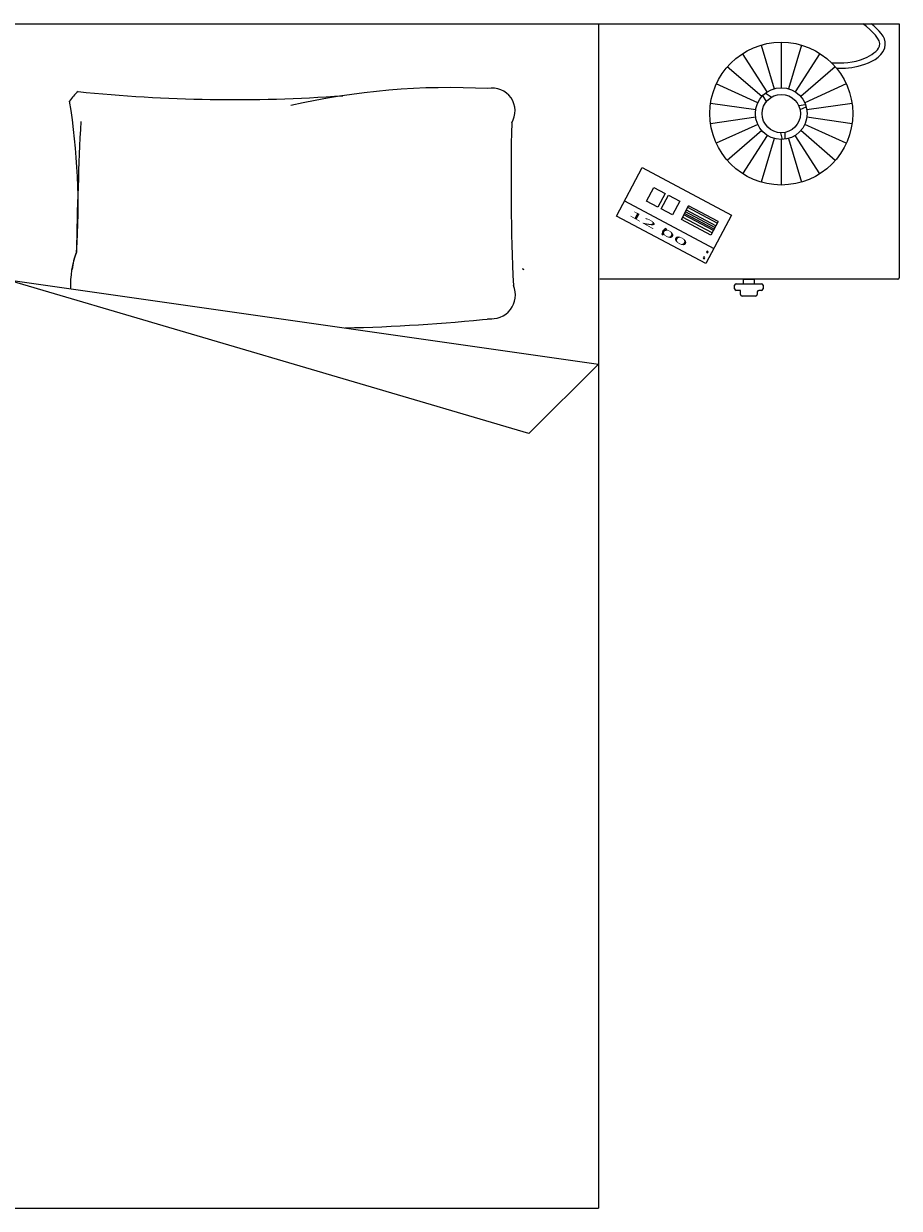
# Model space of a CAD drawing. Units: inches. Extents: x 1994 to 3075, y 3517 to 3950.
# Tile 8 of 58: x 1994.05149 to 1994.10437, y 3553.70967 to 3553.78125. Entities that reach past the tile are written whole.
import ezdxf

# ---------------------------------------------------------------- set-up
doc = ezdxf.new("R2010")
doc.units = ezdxf.units.IN
doc.layers.add('A-FURN-REFR', color=8, linetype='Continuous', lineweight=13)
doc.layers.add('A-FURN-REFR-TEXT', color=7, linetype='Continuous', lineweight=13)
doc.styles.get("Standard").update_dxf_attribs({"font": 'arial.ttf'})

msp = doc.modelspace()

# ---------------------------------------------------------------- linework, layer by layer
at = {"layer": 'A-FURN-REFR'}
for p, q in [((1994.014615338393, 3553.781253037129), (1994.086197299739, 3553.781253037129)), ((1994.086197299739, 3553.781253037129), (1994.10437051092, 3553.781253037129)), ((1994.086197299739, 3553.781253037129), (1994.10437051092, 3553.781253037129)), ((1994.086197299739, 3553.781253037129), (1994.086197299739, 3553.709671075784)), ((1994.10437051092, 3553.781253037129), (1994.10437051092, 3553.76590291077)), ((1994.096027345216, 3553.77996234353), (1994.096802931697, 3553.77732093855)), ((1994.097243416193, 3553.78013718814), (1994.097243416193, 3553.777384270659)), ((1994.097243416193, 3553.78013718814), (1994.097243416193, 3553.777384270659)), ((1994.098459487171, 3553.77996234353), (1994.09768390069, 3553.77732093855)), ((1994.096398132634, 3553.777136073012), (1994.094909793077, 3553.779451974569)), ((1994.09957703931, 3553.779451974569), (1994.098088699753, 3553.777136073012)), ((1994.096061813419, 3553.776844650753), (1994.093981297204, 3553.778647428315)), ((1994.100505535183, 3553.778647428315), (1994.098425018968, 3553.776844650753)), ((1994.095821220632, 3553.776470281071), (1994.093317078811, 3553.777613884321)), ((1994.101169753576, 3553.777613884321), (1994.098665611754, 3553.776470281071)), ((1994.096348791161, 3553.776556785599), (1994.096124540409, 3553.776912848794)), ((1994.096631392656, 3553.776804389888), (1994.096273766541, 3553.777047270305)), ((1994.095695845673, 3553.77604329317), (1994.092970948922, 3553.776435074175)), ((1994.098295634803, 3553.776305435665), (1994.09870586394, 3553.776373715132)), ((1994.098374763921, 3553.776069987851), (1994.098750731625, 3553.776236098163)), ((1994.101515883465, 3553.776435074175), (1994.098790986714, 3553.77604329317)), ((1994.095695845673, 3553.775598279071), (1994.092970948922, 3553.775206498065)), ((1994.101515883465, 3553.775206498065), (1994.098790986714, 3553.775598279071)), ((1994.095821220632, 3553.77517129117), (1994.093317078811, 3553.774027687919)), ((1994.096061813419, 3553.774796921488), (1994.093981297204, 3553.772994143925)), ((1994.097185694303, 3553.774663756577), (1994.097287689547, 3553.774257928554)), ((1994.097453979065, 3553.77468161429), (1994.097451131084, 3553.774271160867)), ((1994.100505535183, 3553.772994143925), (1994.098425018968, 3553.774796921488)), ((1994.101169753576, 3553.774027687919), (1994.098665611754, 3553.77517129117)), ((1994.096398132634, 3553.774505499229), (1994.094909793077, 3553.772189597672)), ((1994.096802931697, 3553.774320633691), (1994.096027345216, 3553.771679228711)), ((1994.097243416193, 3553.774257301582), (1994.097243416193, 3553.7715043841)), ((1994.097243416193, 3553.774257301582), (1994.097243416193, 3553.7715043841)), ((1994.09768390069, 3553.774320633691), (1994.098459487171, 3553.771679228711)), ((1994.09957703931, 3553.772189597672), (1994.098088699753, 3553.774505499229)), ((1994.087280373243, 3553.769626311377), (1994.08883500194, 3553.772558926662)), ((1994.08883500194, 3553.772558926662), (1994.094244007582, 3553.769691521777)), ((1994.08911124464, 3553.770534110705), (1994.089548856707, 3553.771359611893)), ((1994.089548856707, 3553.771359611893), (1994.090232790279, 3553.770997047201)), ((1994.090232790279, 3553.770997047201), (1994.089795178212, 3553.770171546013)), ((1994.087764995145, 3553.770540490821), (1994.093174000788, 3553.767673085936)), ((1994.089795178212, 3553.770171546013), (1994.08911124464, 3553.770534110705)), ((1994.08999172046, 3553.770067355661), (1994.090429332526, 3553.770892856849)), ((1994.090429332526, 3553.770892856849), (1994.091113266099, 3553.770530292157)), ((1994.091113266099, 3553.770530292157), (1994.090675654032, 3553.769704790968)), ((1994.091206990822, 3553.769423120397), (1994.091644602889, 3553.770248621586)), ((1994.0934304468, 3553.769301915686), (1994.091644602889, 3553.770248621586)), ((1994.092689378886, 3553.766758906493), (1994.087280373243, 3553.769626311377)), ((1994.090675654032, 3553.769704790968), (1994.08999172046, 3553.770067355661)), ((1994.093069083129, 3553.76862024769), (1994.091283239217, 3553.76956695359)), ((1994.093139538959, 3553.768753153923), (1994.091353695047, 3553.769699859824)), ((1994.093184219429, 3553.76883743812), (1994.091398375518, 3553.76978414402)), ((1994.093236202765, 3553.768935498271), (1994.091450358854, 3553.769882204172)), ((1994.093295488085, 3553.769047332715), (1994.091509644174, 3553.769994038616)), ((1994.093378615384, 3553.769204142112), (1994.091592771473, 3553.770150848011)), ((1994.094244007582, 3553.769691521777), (1994.092689378886, 3553.766758906493)), ((1994.092992834733, 3553.768476414498), (1994.091206990822, 3553.769423120397)), ((1994.0934304468, 3553.769301915686), (1994.092992834733, 3553.768476414498)), ((1994.08200406422, 3553.75649981287), (1994.050406319066, 3553.765802591595)), ((1994.050406319066, 3553.765802591595), (1994.086197299739, 3553.760685088365)), ((1994.104276005761, 3553.765808405612), (1994.086291804897, 3553.765808405612)), ((1994.094422179853, 3553.765232771723), (1994.094422179853, 3553.76544338097)), ((1994.094516685011, 3553.765537886128), (1994.096051125648, 3553.765537886128)), ((1994.094964999927, 3553.765537886128), (1994.094964999927, 3553.765808405612)), ((1994.094964999927, 3553.765808405612), (1994.095602810732, 3553.765808405612)), ((1994.095602810732, 3553.765808405612), (1994.095602810732, 3553.765537886128)), ((1994.096145630806, 3553.76544338097), (1994.096145630806, 3553.765232771723)), ((1994.094778748834, 3553.765138266565), (1994.094516685011, 3553.765138266565)), ((1994.094778748834, 3553.764886505597), (1994.094778748834, 3553.765138266565)), ((1994.095694556666, 3553.764792000439), (1994.094873253992, 3553.764792000439)), ((1994.095789061825, 3553.765043761406), (1994.095789061825, 3553.764886505597)), ((1994.096051125648, 3553.765138266565), (1994.095883566983, 3553.765138266565)), ((1994.086197299739, 3553.760685088365), (1994.08200406422, 3553.75649981287)), ((1994.050406319066, 3553.709671075784), (1994.086197299739, 3553.709671075784))]:
    msp.add_line(p, q, dxfattribs=at)
for radius in [0.0043164020201009, 0.0015634845390022, 0.0011584684638608]:
    msp.add_circle((1994.097243416193, 3553.77582078612), radius, dxfattribs=at)
for centre, radius, start, end in [((1994.077235901553, 3553.734483994565), 0.0429084957526809, 86.95116779437247, 102.9436181480606), ((1994.077235901553, 3553.734483994565), 0.0429084957526809, 86.95116779437247, 102.9436181480606), ((1994.056131881007, 3553.775420839276), 0.0022014214560216, 128.2265150282699, 148.494767022099), ((1994.064189538159, 3553.868245315502), 0.0915808457167237, 264.0962213920954, 274.1101837577289), ((1994.056131881007, 3553.775420839276), 0.0022014214560216, 41.34610269374063, 41.85120163623711), ((1994.079787317332, 3553.775980935697), 0.0013773909862166, 328.3905013142218, 101.2722137646884), ((1994.079787317332, 3553.775980935697), 0.0013773909862166, 328.3905013142218, 101.2722137646884), ((1994.015816589906, 3553.77023841821), 0.0389565590981439, 355.8780712198786, 9.355599321011619), ((1994.290684928807, 3553.763678902525), 0.2360424856482679, 177.165935704135, 179.0874355336048), ((1994.222820540386, 3553.771782725423), 0.1419027684597849, 178.596248435079, 182.5666707358656), ((1994.222820540386, 3553.771782725423), 0.1419027684597849, 178.596248435079, 182.5666707358656), ((1994.090250464166, 3553.768824155596), 5.53897148363e-05, 90, 270), ((1994.090250464166, 3553.768824155596), 5.53897148363e-05, 270, 90), ((1994.090078349217, 3553.768544240551), 5.53897148363e-05, 90, 270), ((1994.090078349217, 3553.768544240551), 5.53897148363e-05, 270, 90), ((1994.059837029154, 3553.765472592822), 0.0055260654244096, 159.1632261124114, 182.3747851250911), ((1994.0572601995, 3553.766265761826), 0.0028410445555686, 155.6256321457925, 177.330230157294), ((1994.092775809128, 3553.767456349182), 5.53897148363e-05, 90, 270), ((1994.092775809128, 3553.767456349182), 5.53897148363e-05, 270, 90), ((1994.09257568141, 3553.767106752659), 5.53897148363e-05, 90, 270), ((1994.09257568141, 3553.767106752659), 5.53897148363e-05, 270, 90), ((1994.081692691451, 3553.766478351356), 7.56041267044e-05, 180, 270), ((1994.079757150556, 3553.76485088119), 0.0014250910037829, 260.3424204380755, 23.89158844542257), ((1994.079757150556, 3553.76485088119), 0.0014250910037829, 260.3424204380755, 23.89158844542257), ((1994.094516685011, 3553.76544338097), 9.45051583805e-05, 90, 180), ((1994.094516685011, 3553.765232771723), 9.45051583805e-05, 180, 270), ((1994.096051125648, 3553.76544338097), 9.45051583805e-05, 0, 90), ((1994.096051125648, 3553.765232771723), 9.45051583805e-05, 270, 0), ((1994.104276005761, 3553.76590291077), 9.45051583805e-05, 270, 0), ((1994.094873253992, 3553.764886505597), 9.45051583805e-05, 180, 270), ((1994.095694556666, 3553.764886505597), 9.45051583805e-05, 270, 0), ((1994.095883566983, 3553.765043761406), 9.45051583805e-05, 90, 180), ((1994.06843228948, 3553.873275096342), 0.1104315287461407, 271.2842077037144, 275.8860860669378), ((1994.06843228948, 3553.873275096342), 0.1104315287461407, 271.2842077037144, 275.8860860669378)]:
    msp.add_arc(centre, radius, start, end, dxfattribs=at)
for points, knots in [([(1994.100280415764, 3553.778888025924), (1994.100933665112, 3553.778875793347), (1994.101956137112, 3553.778868956396), (1994.103683291971, 3553.77999348335), (1994.102739600918, 3553.780785400519), (1994.102174151574, 3553.781253037129)], [0, 0, 0, 0, 0.0020194675198324, 0.0031659294015444, 0.0048546887782932, 0.0048546887782932, 0.0048546887782932, 0.0048546887782932]), ([(1994.100581058264, 3553.778557841438), (1994.101053307834, 3553.778553992103), (1994.101554545229, 3553.778574259315), (1994.10262119447, 3553.778907428329), (1994.103293277311, 3553.779159156177), (1994.103655051326, 3553.780313714741), (1994.103255082035, 3553.78073398885), (1994.10280946264, 3553.781141867933), (1994.102745871023, 3553.781197724685), (1994.102681356186, 3553.781253037129)], [0.0077183477163671, 0.0077183477163671, 0.0077183477163671, 0.0077183477163671, 0.0428867239757183, 0.0428867239757183, 0.0785443346356031, 0.0785443346356031, 0.1084777623087474, 0.1084777623087474, 0.1132872864949097, 0.1132872864949097, 0.1132872864949097, 0.1132872864949097])]:
    msp.add_open_spline(points, degree=3, knots=knots, dxfattribs=at)

# ---------------------------------------------------------------- texts
at = {"layer": 'A-FURN-REFR-TEXT', "width": 3}
msp.add_text('12 00', height=0.000395772154613, rotation=330.6435157060532, dxfattribs=at).set_placement((1994.088007371235, 3553.769679963318))

doc.saveas('drawing.dxf')
